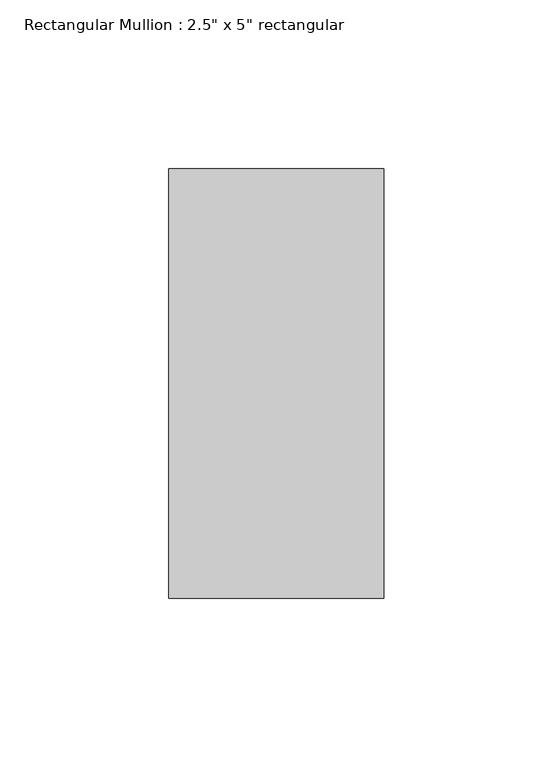
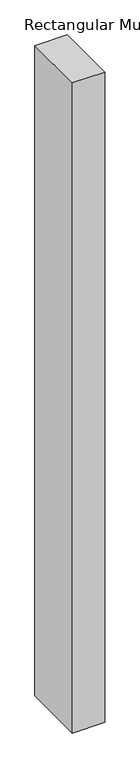
"""IFC4 building model written with IfcOpenShell, lengths in millimetres: member geometry."""

from ifc_helpers import new_model, si_unit, frame, origin, place, context, project, spatial, polyline, outline, extrude, source, transform, mapped, element, save


def member_10605c90(model_context):
    return source(origin(), model_context, "Body", "SweptSolid", [
        extrude(outline(polyline([(0.0, 63.5), (0.0, -63.5), (-63.5, -63.5), (-63.5, 63.5), (0.0, 63.5)])), frame((0.0, 0.0, -1341.9666665), z_axis=(0.0, 0.0, 1.0), x_axis=(1.0, 0.0, 0.0)), (0.0, 0.0, 1.0), 1341.9666665),
    ])


if __name__ == "__main__":
    model = new_model("IFC4")
    model_context = context("Model", 3, world=origin())
    ifc_project = project(units=[si_unit("LENGTHUNIT", "METRE", prefix="MILLI")], contexts=[model_context])
    site = spatial("IfcSite", under=ifc_project)
    building = spatial("IfcBuilding", under=site)
    placement = place(None, origin())
    member_shape = member_10605c90(model_context)
    element("IfcMember", 1, ObjectType="Rectangular Mullion : 2.5\" x 5\" rectangular", at=placement, inside=building, context=model_context, shape_type="MappedRepresentation", body=[
        mapped(member_shape, transform((0.0, 0.0, 0.0), x_axis=(1.0, 0.0, 0.0), y_axis=(0.0, 1.0, 0.0), z_axis=(0.0, 0.0, 1.0))),
    ])
    save(model, "model.ifc")

# Revit data of these elements
# Type "Rectangular Mullion : 2.5\" x 5\" rectangular"
#   built-in parameter 1007304 = 0.416667 (stored number, unit not read)
#   built-in parameter 1007301 = 0.104167 (stored number, unit not read)
#   built-in parameter 1007300 = 0.104167 (stored number, unit not read)
# Element 1 (IfcMember, "Rectangular Mullion : 2.5\" x 5\" rectangular")
#   Materials on its faces: "Aluminum"
# Materials
#   "Aluminum": class "Metal", colour RGB 247 247 247, transparency 0, Description = "Aluminum 6061", Cost = 0
